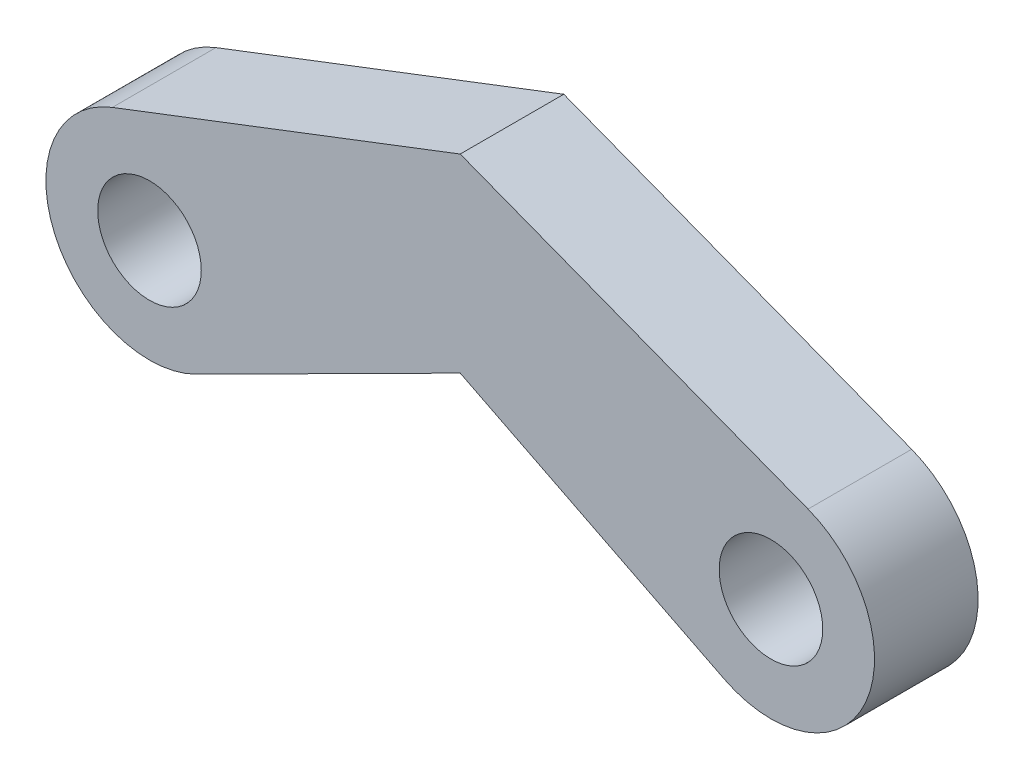
ISO-10303-21;
HEADER;
FILE_DESCRIPTION(('STEP AP214'),'2;1');
FILE_NAME('part.step','',(''),(''),'','','');
FILE_SCHEMA(('AUTOMOTIVE_DESIGN { 1 0 10303 214 1 1 1 1 }'));
ENDSEC;
DATA;
#1=APPLICATION_CONTEXT('core data for automotive mechanical design processes');
#2=APPLICATION_PROTOCOL_DEFINITION('international standard','automotive_design',2000,#1);
#3=PRODUCT_CONTEXT('',#1,'mechanical');
#4=PRODUCT('Part','Part','',(#3));
#5=PRODUCT_RELATED_PRODUCT_CATEGORY('part','',(#4));
#6=PRODUCT_DEFINITION_FORMATION('','',#4);
#7=PRODUCT_DEFINITION_CONTEXT('part definition',#1,'design');
#8=PRODUCT_DEFINITION('design','',#6,#7);
#9=PRODUCT_DEFINITION_SHAPE('','',#8);
#10=(LENGTH_UNIT() NAMED_UNIT(*) SI_UNIT(.MILLI.,.METRE.));
#11=(NAMED_UNIT(*) PLANE_ANGLE_UNIT() SI_UNIT($,.RADIAN.));
#12=(NAMED_UNIT(*) SI_UNIT($,.STERADIAN.) SOLID_ANGLE_UNIT());
#13=UNCERTAINTY_MEASURE_WITH_UNIT(LENGTH_MEASURE(1.E-05),#10,'distance_accuracy_value','');
#14=(GEOMETRIC_REPRESENTATION_CONTEXT(3) GLOBAL_UNCERTAINTY_ASSIGNED_CONTEXT((#13)) GLOBAL_UNIT_ASSIGNED_CONTEXT((#10,
#11,#12)) REPRESENTATION_CONTEXT('',''));
#15=CARTESIAN_POINT('',(0.,0.,0.));
#16=DIRECTION('',(0.,0.,1.));
#17=DIRECTION('',(1.,0.,0.));
#18=AXIS2_PLACEMENT_3D('',#15,#16,#17);
#19=CARTESIAN_POINT('',(-19.05,-8.39938057701995,-6.35));
#20=DIRECTION('',(0.,0.,1.));
#21=DIRECTION('',(1.,0.,0.));
#22=AXIS2_PLACEMENT_3D('',#19,#20,#21);
#23=CYLINDRICAL_SURFACE('',#22,6.35);
#24=CARTESIAN_POINT('',(-19.05,-8.39938057701995,0.));
#25=DIRECTION('',(0.,0.,1.));
#26=DIRECTION('',(1.,0.,0.));
#27=AXIS2_PLACEMENT_3D('',#24,#25,#26);
#28=CIRCLE('',#27,6.35);
#29=CARTESIAN_POINT('',(-21.3256364796127,-2.47114486876273,0.));
#30=VERTEX_POINT('',#29);
#31=CARTESIAN_POINT('',(-16.1942804190222,-14.0710087096482,0.));
#32=VERTEX_POINT('',#31);
#33=EDGE_CURVE('E126',#30,#32,#28,.T.);
#34=ORIENTED_EDGE('',*,*,#33,.F.);
#35=DIRECTION('',(0.,0.,1.));
#36=VECTOR('',#35,1.);
#37=CARTESIAN_POINT('',(-21.3256364796127,-2.47114486876273,-6.35));
#38=LINE('',#37,#36);
#39=CARTESIAN_POINT('',(-21.3256364796127,-2.47114486876273,-6.35));
#40=VERTEX_POINT('',#39);
#41=EDGE_CURVE('E11',#40,#30,#38,.T.);
#42=ORIENTED_EDGE('',*,*,#41,.F.);
#43=CARTESIAN_POINT('',(-19.05,-8.39938057701995,-6.35));
#44=DIRECTION('',(0.,0.,1.));
#45=DIRECTION('',(1.,0.,0.));
#46=AXIS2_PLACEMENT_3D('',#43,#44,#45);
#47=CIRCLE('',#46,6.35);
#48=CARTESIAN_POINT('',(-16.1942804190222,-14.0710087096482,-6.35));
#49=VERTEX_POINT('',#48);
#50=EDGE_CURVE('E141',#40,#49,#47,.T.);
#51=ORIENTED_EDGE('',*,*,#50,.T.);
#52=DIRECTION('',(0.,0.,1.));
#53=VECTOR('',#52,1.);
#54=CARTESIAN_POINT('',(-16.1942804190222,-14.0710087096482,-6.35));
#55=LINE('',#54,#53);
#56=EDGE_CURVE('E46',#49,#32,#55,.T.);
#57=ORIENTED_EDGE('',*,*,#56,.T.);
#58=EDGE_LOOP('',(#34,#42,#51,#57));
#59=FACE_BOUND('',#58,.T.);
#60=ADVANCED_FACE('F43',(#59),#23,.T.);
#61=CARTESIAN_POINT('',(-21.3256364796127,-2.47114486876273,-6.35));
#62=DIRECTION('',(-0.358367949545306,0.9335804264972,0.));
#63=DIRECTION('',(-0.9335804264972,-0.358367949545306,0.));
#64=AXIS2_PLACEMENT_3D('',#61,#62,#63);
#65=PLANE('',#64);
#66=DIRECTION('',(-0.9335804264972,-0.358367949545306,0.));
#67=VECTOR('',#66,1.);
#68=CARTESIAN_POINT('',(-21.3256364796127,-2.47114486876273,0.));
#69=LINE('',#68,#67);
#70=CARTESIAN_POINT('',(0.,5.715,0.));
#71=VERTEX_POINT('',#70);
#72=EDGE_CURVE('E143',#71,#30,#69,.T.);
#73=ORIENTED_EDGE('',*,*,#72,.F.);
#74=DIRECTION('',(0.,0.,1.));
#75=VECTOR('',#74,1.);
#76=CARTESIAN_POINT('',(0.,5.715,-6.35));
#77=LINE('',#76,#75);
#78=CARTESIAN_POINT('',(0.,5.715,-6.35));
#79=VERTEX_POINT('',#78);
#80=EDGE_CURVE('E55',#79,#71,#77,.T.);
#81=ORIENTED_EDGE('',*,*,#80,.F.);
#82=DIRECTION('',(-0.9335804264972,-0.358367949545306,0.));
#83=VECTOR('',#82,1.);
#84=CARTESIAN_POINT('',(-21.3256364796127,-2.47114486876273,-6.35));
#85=LINE('',#84,#83);
#86=EDGE_CURVE('E120',#79,#40,#85,.T.);
#87=ORIENTED_EDGE('',*,*,#86,.T.);
#88=ORIENTED_EDGE('',*,*,#41,.T.);
#89=EDGE_LOOP('',(#73,#81,#87,#88));
#90=FACE_BOUND('',#89,.T.);
#91=ADVANCED_FACE('F151',(#90),#65,.T.);
#92=CARTESIAN_POINT('',(0.,5.715,-6.35));
#93=DIRECTION('',(0.358367949545304,0.9335804264972,0.));
#94=DIRECTION('',(-0.9335804264972,0.358367949545304,0.));
#95=AXIS2_PLACEMENT_3D('',#92,#93,#94);
#96=PLANE('',#95);
#97=DIRECTION('',(-0.9335804264972,0.358367949545304,0.));
#98=VECTOR('',#97,1.);
#99=CARTESIAN_POINT('',(0.,5.715,0.));
#100=LINE('',#99,#98);
#101=CARTESIAN_POINT('',(21.3256364796127,-2.4711448687627,0.));
#102=VERTEX_POINT('',#101);
#103=EDGE_CURVE('E104',#102,#71,#100,.T.);
#104=ORIENTED_EDGE('',*,*,#103,.F.);
#105=DIRECTION('',(0.,0.,1.));
#106=VECTOR('',#105,1.);
#107=CARTESIAN_POINT('',(21.3256364796127,-2.4711448687627,-6.35));
#108=LINE('',#107,#106);
#109=CARTESIAN_POINT('',(21.3256364796127,-2.4711448687627,-6.35));
#110=VERTEX_POINT('',#109);
#111=EDGE_CURVE('E99',#110,#102,#108,.T.);
#112=ORIENTED_EDGE('',*,*,#111,.F.);
#113=DIRECTION('',(-0.9335804264972,0.358367949545304,0.));
#114=VECTOR('',#113,1.);
#115=CARTESIAN_POINT('',(0.,5.715,-6.35));
#116=LINE('',#115,#114);
#117=EDGE_CURVE('E103',#110,#79,#116,.T.);
#118=ORIENTED_EDGE('',*,*,#117,.T.);
#119=ORIENTED_EDGE('',*,*,#80,.T.);
#120=EDGE_LOOP('',(#104,#112,#118,#119));
#121=FACE_BOUND('',#120,.T.);
#122=ADVANCED_FACE('F105',(#121),#96,.T.);
#123=CARTESIAN_POINT('',(19.05,-8.39938057701991,-6.35));
#124=DIRECTION('',(0.,0.,1.));
#125=DIRECTION('',(1.,0.,0.));
#126=AXIS2_PLACEMENT_3D('',#123,#124,#125);
#127=CYLINDRICAL_SURFACE('',#126,6.34999999999999);
#128=CARTESIAN_POINT('',(19.05,-8.39938057701991,0.));
#129=DIRECTION('',(0.,0.,1.));
#130=DIRECTION('',(1.,0.,0.));
#131=AXIS2_PLACEMENT_3D('',#128,#129,#130);
#132=CIRCLE('',#131,6.34999999999999);
#133=CARTESIAN_POINT('',(16.1942804190222,-14.0710087096481,0.));
#134=VERTEX_POINT('',#133);
#135=EDGE_CURVE('E137',#134,#102,#132,.T.);
#136=ORIENTED_EDGE('',*,*,#135,.F.);
#137=DIRECTION('',(0.,0.,1.));
#138=VECTOR('',#137,1.);
#139=CARTESIAN_POINT('',(16.1942804190222,-14.0710087096481,-6.35));
#140=LINE('',#139,#138);
#141=CARTESIAN_POINT('',(16.1942804190222,-14.0710087096481,-6.35));
#142=VERTEX_POINT('',#141);
#143=EDGE_CURVE('E109',#142,#134,#140,.T.);
#144=ORIENTED_EDGE('',*,*,#143,.F.);
#145=CARTESIAN_POINT('',(19.05,-8.39938057701991,-6.35));
#146=DIRECTION('',(0.,0.,1.));
#147=DIRECTION('',(1.,0.,0.));
#148=AXIS2_PLACEMENT_3D('',#145,#146,#147);
#149=CIRCLE('',#148,6.34999999999999);
#150=EDGE_CURVE('E119',#142,#110,#149,.T.);
#151=ORIENTED_EDGE('',*,*,#150,.T.);
#152=ORIENTED_EDGE('',*,*,#111,.T.);
#153=EDGE_LOOP('',(#136,#144,#151,#152));
#154=FACE_BOUND('',#153,.T.);
#155=ADVANCED_FACE('F117',(#154),#127,.T.);
#156=CARTESIAN_POINT('',(0.,-5.91703200119698,-6.35));
#157=DIRECTION('',(-0.44971961905162,-0.893169784665864,0.));
#158=DIRECTION('',(0.893169784665864,-0.44971961905162,0.));
#159=AXIS2_PLACEMENT_3D('',#156,#157,#158);
#160=PLANE('',#159);
#161=DIRECTION('',(0.893169784665864,-0.44971961905162,0.));
#162=VECTOR('',#161,1.);
#163=CARTESIAN_POINT('',(0.,-5.91703200119698,0.));
#164=LINE('',#163,#162);
#165=CARTESIAN_POINT('',(0.,-5.91703200119698,0.));
#166=VERTEX_POINT('',#165);
#167=EDGE_CURVE('E132',#166,#134,#164,.T.);
#168=ORIENTED_EDGE('',*,*,#167,.F.);
#169=DIRECTION('',(0.,0.,1.));
#170=VECTOR('',#169,1.);
#171=CARTESIAN_POINT('',(0.,-5.91703200119698,-6.35));
#172=LINE('',#171,#170);
#173=CARTESIAN_POINT('',(0.,-5.91703200119698,-6.35));
#174=VERTEX_POINT('',#173);
#175=EDGE_CURVE('E148',#174,#166,#172,.T.);
#176=ORIENTED_EDGE('',*,*,#175,.F.);
#177=DIRECTION('',(0.893169784665864,-0.44971961905162,0.));
#178=VECTOR('',#177,1.);
#179=CARTESIAN_POINT('',(0.,-5.91703200119698,-6.35));
#180=LINE('',#179,#178);
#181=EDGE_CURVE('E121',#174,#142,#180,.T.);
#182=ORIENTED_EDGE('',*,*,#181,.T.);
#183=ORIENTED_EDGE('',*,*,#143,.T.);
#184=EDGE_LOOP('',(#168,#176,#182,#183));
#185=FACE_BOUND('',#184,.T.);
#186=ADVANCED_FACE('F163',(#185),#160,.T.);
#187=CARTESIAN_POINT('',(-16.1942804190222,-14.0710087096482,-6.35));
#188=DIRECTION('',(0.449719619051623,-0.893169784665862,0.));
#189=DIRECTION('',(0.893169784665862,0.449719619051623,0.));
#190=AXIS2_PLACEMENT_3D('',#187,#188,#189);
#191=PLANE('',#190);
#192=DIRECTION('',(0.893169784665862,0.449719619051623,0.));
#193=VECTOR('',#192,1.);
#194=CARTESIAN_POINT('',(-16.1942804190222,-14.0710087096482,0.));
#195=LINE('',#194,#193);
#196=EDGE_CURVE('E134',#32,#166,#195,.T.);
#197=ORIENTED_EDGE('',*,*,#196,.F.);
#198=ORIENTED_EDGE('',*,*,#56,.F.);
#199=DIRECTION('',(0.893169784665862,0.449719619051623,0.));
#200=VECTOR('',#199,1.);
#201=CARTESIAN_POINT('',(-16.1942804190222,-14.0710087096482,-6.35));
#202=LINE('',#201,#200);
#203=EDGE_CURVE('E124',#49,#174,#202,.T.);
#204=ORIENTED_EDGE('',*,*,#203,.T.);
#205=ORIENTED_EDGE('',*,*,#175,.T.);
#206=EDGE_LOOP('',(#197,#198,#204,#205));
#207=FACE_BOUND('',#206,.T.);
#208=ADVANCED_FACE('F146',(#207),#191,.T.);
#209=CARTESIAN_POINT('',(-19.05,-8.39938057701995,-6.35));
#210=DIRECTION('',(0.,0.,1.));
#211=DIRECTION('',(1.,0.,0.));
#212=AXIS2_PLACEMENT_3D('',#209,#210,#211);
#213=PLANE('',#212);
#214=CARTESIAN_POINT('',(19.05,-8.39938057701991,-6.35));
#215=DIRECTION('',(0.,0.,1.));
#216=DIRECTION('',(1.,0.,0.));
#217=AXIS2_PLACEMENT_3D('',#214,#215,#216);
#218=CIRCLE('',#217,3.175);
#219=CARTESIAN_POINT('',(22.225,-8.39938057701991,-6.35));
#220=VERTEX_POINT('',#219);
#221=EDGE_CURVE('E187',#220,#220,#218,.T.);
#222=ORIENTED_EDGE('',*,*,#221,.T.);
#223=EDGE_LOOP('',(#222));
#224=FACE_BOUND('',#223,.T.);
#225=CARTESIAN_POINT('',(-19.05,-8.39938057701995,-6.35));
#226=DIRECTION('',(0.,0.,1.));
#227=DIRECTION('',(1.,0.,0.));
#228=AXIS2_PLACEMENT_3D('',#225,#226,#227);
#229=CIRCLE('',#228,3.175);
#230=CARTESIAN_POINT('',(-15.875,-8.39938057701995,-6.35));
#231=VERTEX_POINT('',#230);
#232=EDGE_CURVE('E131',#231,#231,#229,.T.);
#233=ORIENTED_EDGE('',*,*,#232,.T.);
#234=EDGE_LOOP('',(#233));
#235=FACE_BOUND('',#234,.T.);
#236=ORIENTED_EDGE('',*,*,#50,.F.);
#237=ORIENTED_EDGE('',*,*,#86,.F.);
#238=ORIENTED_EDGE('',*,*,#117,.F.);
#239=ORIENTED_EDGE('',*,*,#150,.F.);
#240=ORIENTED_EDGE('',*,*,#181,.F.);
#241=ORIENTED_EDGE('',*,*,#203,.F.);
#242=EDGE_LOOP('',(#236,#237,#238,#239,#240,#241));
#243=FACE_BOUND('',#242,.T.);
#244=ADVANCED_FACE('F111',(#224,#235,#243),#213,.F.);
#245=CARTESIAN_POINT('',(-19.05,-8.39938057701995,0.));
#246=DIRECTION('',(0.,0.,1.));
#247=DIRECTION('',(1.,0.,0.));
#248=AXIS2_PLACEMENT_3D('',#245,#246,#247);
#249=PLANE('',#248);
#250=CARTESIAN_POINT('',(19.05,-8.39938057701991,0.));
#251=DIRECTION('',(0.,0.,1.));
#252=DIRECTION('',(1.,0.,0.));
#253=AXIS2_PLACEMENT_3D('',#250,#251,#252);
#254=CIRCLE('',#253,3.175);
#255=CARTESIAN_POINT('',(22.225,-8.39938057701991,0.));
#256=VERTEX_POINT('',#255);
#257=EDGE_CURVE('E192',#256,#256,#254,.T.);
#258=ORIENTED_EDGE('',*,*,#257,.F.);
#259=EDGE_LOOP('',(#258));
#260=FACE_BOUND('',#259,.T.);
#261=CARTESIAN_POINT('',(-19.05,-8.39938057701995,0.));
#262=DIRECTION('',(0.,0.,1.));
#263=DIRECTION('',(1.,0.,0.));
#264=AXIS2_PLACEMENT_3D('',#261,#262,#263);
#265=CIRCLE('',#264,3.175);
#266=CARTESIAN_POINT('',(-15.875,-8.39938057701995,0.));
#267=VERTEX_POINT('',#266);
#268=EDGE_CURVE('E191',#267,#267,#265,.T.);
#269=ORIENTED_EDGE('',*,*,#268,.F.);
#270=EDGE_LOOP('',(#269));
#271=FACE_BOUND('',#270,.T.);
#272=ORIENTED_EDGE('',*,*,#33,.T.);
#273=ORIENTED_EDGE('',*,*,#196,.T.);
#274=ORIENTED_EDGE('',*,*,#167,.T.);
#275=ORIENTED_EDGE('',*,*,#135,.T.);
#276=ORIENTED_EDGE('',*,*,#103,.T.);
#277=ORIENTED_EDGE('',*,*,#72,.T.);
#278=EDGE_LOOP('',(#272,#273,#274,#275,#276,#277));
#279=FACE_BOUND('',#278,.T.);
#280=ADVANCED_FACE('F147',(#260,#271,#279),#249,.T.);
#281=CARTESIAN_POINT('',(-19.05,-8.39938057701995,-6.35));
#282=DIRECTION('',(0.,0.,1.));
#283=DIRECTION('',(1.,0.,0.));
#284=AXIS2_PLACEMENT_3D('',#281,#282,#283);
#285=CYLINDRICAL_SURFACE('',#284,3.175);
#286=ORIENTED_EDGE('',*,*,#232,.F.);
#287=EDGE_LOOP('',(#286));
#288=FACE_BOUND('',#287,.T.);
#289=ORIENTED_EDGE('',*,*,#268,.T.);
#290=EDGE_LOOP('',(#289));
#291=FACE_BOUND('',#290,.T.);
#292=ADVANCED_FACE('F172',(#288,#291),#285,.F.);
#293=CARTESIAN_POINT('',(19.05,-8.39938057701991,-6.35));
#294=DIRECTION('',(0.,0.,1.));
#295=DIRECTION('',(1.,0.,0.));
#296=AXIS2_PLACEMENT_3D('',#293,#294,#295);
#297=CYLINDRICAL_SURFACE('',#296,3.175);
#298=ORIENTED_EDGE('',*,*,#221,.F.);
#299=EDGE_LOOP('',(#298));
#300=FACE_BOUND('',#299,.T.);
#301=ORIENTED_EDGE('',*,*,#257,.T.);
#302=EDGE_LOOP('',(#301));
#303=FACE_BOUND('',#302,.T.);
#304=ADVANCED_FACE('F185',(#300,#303),#297,.F.);
#305=CLOSED_SHELL('',(#60,#91,#122,#155,#186,#208,#244,#280,#292,#304));
#306=MANIFOLD_SOLID_BREP('B2',#305);
#307=ADVANCED_BREP_SHAPE_REPRESENTATION('',(#18,#306),#14);
#308=SHAPE_DEFINITION_REPRESENTATION(#9,#307);
ENDSEC;
END-ISO-10303-21;
